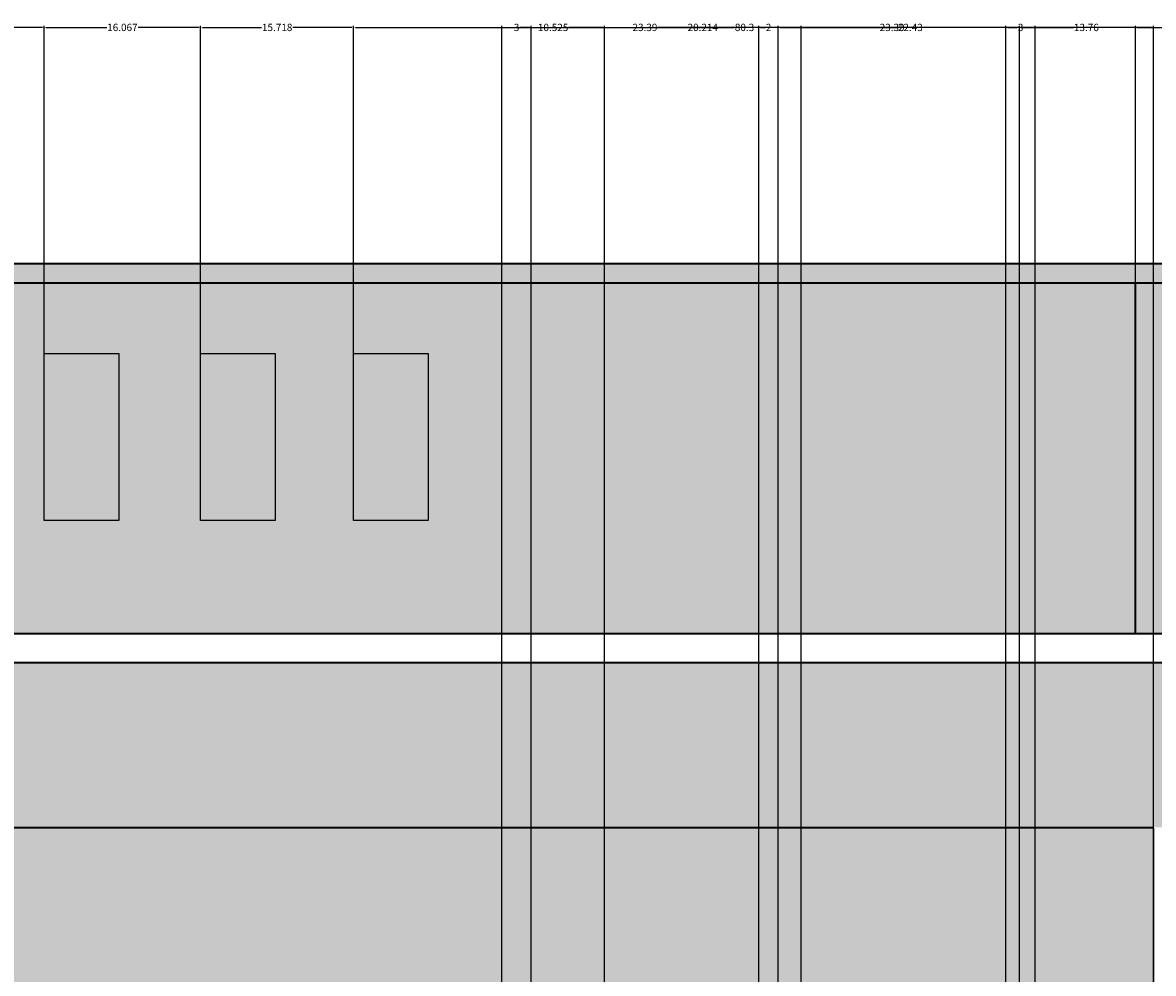
# Model space of a CAD drawing. Units: inches. Extents: x 62 to 566, y 66 to 528.
# Tile 10 of 20: x 168 to 284, y 430 to 528. Entities that reach past the tile are written whole.
import ezdxf

# ---------------------------------------------------------------- set-up
doc = ezdxf.new("R2010")
doc.units = ezdxf.units.IN
doc.header["$MEASUREMENT"] = 0
for name, color, linetype, lineweight in [('A-ANNO-DIMS', 2, 'Continuous', 18), ('A-ELEV', 7, 'Continuous', 35), ('A-GLAZ', 3, 'Continuous', 25), ('A-WALL-PATT', 8, 'Continuous', 13)]:
    doc.layers.add(name, color=color, linetype=linetype, lineweight=lineweight)
doc.styles.get("Standard").update_dxf_attribs({"font": 'arial.ttf'})
doc.dimstyles.get("Standard").update_dxf_attribs({"dimtxt": 0.75, "dimasz": 0.18, "dimexe": 0.18, "dimexo": 0.0625, "dimgap": 0.09, "dimtad": 0, "dimtih": 1, "dimtoh": 1, "dimdec": 4, "dimzin": 0, "dimdsep": 46, "dimlunit": 4, "dimtxsty": 'Standard', "dimcen": 0.09, "dimadec": 0, "dimazin": 0, "dimtfac": 1, "dimtdec": 4, "dimtofl": 0, "dimtmove": 0, "dimatfit": 3, "dimfxl": 1, "dimtolj": 1, "dimtzin": 0, "dimarcsym": 0})

# ---------------------------------------------------------------- blocks, each defined once
blk = doc.blocks.new('VENT-OPENING')
blk.add_lwpolyline([(0, 17.13), (7.66, 17.13), (7.66, 0), (0, 0)], close=True)
blk = doc.blocks.new('*D28')
at = {"layer": 'A-ANNO-DIMS', "color": 0, "lineweight": -2, "transparency": 16777216}
for p, q in [((155.59, 493.49), (155.59, 527.47)), ((170.26, 493.84), (170.26, 527.47)), ((155.77, 527.29), (161.61, 527.29)), ((170.08, 527.29), (164.25, 527.29))]:
    blk.add_line(p, q, dxfattribs=at)
at = {"layer": 'A-ANNO-DIMS', "color": 0, "transparency": 16777216}
for points in [[(155.77, 527.32), (155.77, 527.26), (155.59, 527.29)], [(170.08, 527.32), (170.08, 527.26), (170.26, 527.29)]]:
    blk.add_solid(points, dxfattribs=at)
at = {"layer": 'Defpoints', "color": 0, "transparency": 16777216}
for p in [(170.26, 527.29), (170.26, 493.78), (155.59, 493.43)]:
    blk.add_point(p, dxfattribs=at)
at = {"layer": 'A-ANNO-DIMS', "color": 0, "transparency": 16777216, "insert": (162.93, 527.29), "char_height": 0.75, "attachment_point": 5}
blk.add_mtext('\\A1;14.67', dxfattribs=at)
blk = doc.blocks.new('*D29')
at = {"layer": 'A-ANNO-DIMS', "color": 0, "lineweight": -2, "transparency": 16777216}
for p, q in [((170.26, 493.84), (170.26, 527.47)), ((186.33, 493.84), (186.33, 527.47)), ((170.44, 527.29), (176.68, 527.29)), ((186.15, 527.29), (179.91, 527.29))]:
    blk.add_line(p, q, dxfattribs=at)
at = {"layer": 'A-ANNO-DIMS', "color": 0, "transparency": 16777216}
for points in [[(170.44, 527.32), (170.44, 527.26), (170.26, 527.29)], [(186.15, 527.32), (186.15, 527.26), (186.33, 527.29)]]:
    blk.add_solid(points, dxfattribs=at)
at = {"layer": 'Defpoints', "color": 0, "transparency": 16777216}
for p in [(186.33, 527.29), (170.26, 493.78), (186.33, 493.78)]:
    blk.add_point(p, dxfattribs=at)
at = {"layer": 'A-ANNO-DIMS', "color": 0, "transparency": 16777216, "insert": (178.29, 527.29), "char_height": 0.75, "attachment_point": 5}
blk.add_mtext('\\A1;16.067', dxfattribs=at)
blk = doc.blocks.new('*D30')
at = {"layer": 'A-ANNO-DIMS', "color": 0, "lineweight": -2, "transparency": 16777216}
for p, q in [((186.33, 493.84), (186.33, 527.47)), ((202.04, 493.84), (202.04, 527.47)), ((186.51, 527.29), (192.57, 527.29)), ((201.86, 527.29), (195.8, 527.29))]:
    blk.add_line(p, q, dxfattribs=at)
at = {"layer": 'A-ANNO-DIMS', "color": 0, "transparency": 16777216}
for points in [[(186.51, 527.32), (186.51, 527.26), (186.33, 527.29)], [(201.86, 527.32), (201.86, 527.26), (202.04, 527.29)]]:
    blk.add_solid(points, dxfattribs=at)
at = {"layer": 'Defpoints', "color": 0, "transparency": 16777216}
for p in [(202.04, 527.29), (186.33, 493.78), (202.04, 493.78)]:
    blk.add_point(p, dxfattribs=at)
at = {"layer": 'A-ANNO-DIMS', "color": 0, "transparency": 16777216, "insert": (194.19, 527.29), "char_height": 0.75, "attachment_point": 5}
blk.add_mtext('\\A1;15.718', dxfattribs=at)
blk = doc.blocks.new('*D31')
at = {"layer": 'A-ANNO-DIMS', "color": 0, "lineweight": -2, "transparency": 16777216}
for p, q in [((202.04, 493.84), (202.04, 527.47)), ((282.35, 501.1), (282.35, 527.47)), ((202.22, 527.29), (241.13, 527.29)), ((282.17, 527.29), (243.26, 527.29))]:
    blk.add_line(p, q, dxfattribs=at)
at = {"layer": 'A-ANNO-DIMS', "color": 0, "transparency": 16777216}
for points in [[(202.22, 527.32), (202.22, 527.26), (202.04, 527.29)], [(282.17, 527.32), (282.17, 527.26), (282.35, 527.29)]]:
    blk.add_solid(points, dxfattribs=at)
at = {"layer": 'Defpoints', "color": 0, "transparency": 16777216}
for p in [(282.35, 527.29), (282.35, 501.04), (202.04, 493.78)]:
    blk.add_point(p, dxfattribs=at)
at = {"layer": 'A-ANNO-DIMS', "color": 0, "transparency": 16777216, "insert": (242.2, 527.29), "char_height": 0.75, "attachment_point": 5}
blk.add_mtext('\\A1;80.3', dxfattribs=at)
blk = doc.blocks.new('*D32')
at = {"layer": 'A-ANNO-DIMS', "color": 0, "lineweight": -2, "transparency": 16777216}
for p, q in [((282.35, 501.1), (282.35, 527.47)), ((416.08, 501.1), (416.08, 527.47)), ((282.53, 527.29), (347.61, 527.29)), ((415.9, 527.29), (350.83, 527.29))]:
    blk.add_line(p, q, dxfattribs=at)
at = {"layer": 'A-ANNO-DIMS', "color": 0, "transparency": 16777216}
for points in [[(282.53, 527.32), (282.53, 527.26), (282.35, 527.29)], [(415.9, 527.32), (415.9, 527.26), (416.08, 527.29)]]:
    blk.add_solid(points, dxfattribs=at)
at = {"layer": 'Defpoints', "color": 0, "transparency": 16777216}
for p in [(416.08, 527.29), (282.35, 501.04), (416.08, 501.04)]:
    blk.add_point(p, dxfattribs=at)
at = {"layer": 'A-ANNO-DIMS', "color": 0, "transparency": 16777216, "insert": (349.22, 527.29), "char_height": 0.75, "attachment_point": 5}
blk.add_mtext('\\A1;133.73', dxfattribs=at)
blk = doc.blocks.new('*D39')
at = {"layer": 'A-ANNO-DIMS', "color": 0, "lineweight": -2, "transparency": 16777216}
for p, q in [((284.2, 445.04), (284.2, 65.94)), ((217.28, 420.53), (217.28, 65.94)), ((217.46, 66.12), (249.38, 66.12)), ((284.02, 66.12), (252.1, 66.12))]:
    blk.add_line(p, q, dxfattribs=at)
at = {"layer": 'A-ANNO-DIMS', "color": 0, "transparency": 16777216}
for points in [[(217.46, 66.15), (217.46, 66.09), (217.28, 66.12)], [(284.02, 66.15), (284.02, 66.09), (284.2, 66.12)]]:
    blk.add_solid(points, dxfattribs=at)
at = {"layer": 'Defpoints', "color": 0, "transparency": 16777216}
for p in [(284.2, 445.11), (217.28, 420.6), (284.2, 66.12)]:
    blk.add_point(p, dxfattribs=at)
at = {"layer": 'A-ANNO-DIMS', "color": 0, "transparency": 16777216, "insert": (250.74, 66.12), "char_height": 0.75, "attachment_point": 5}
blk.add_mtext('\\A1;66.93', dxfattribs=at)
blk = doc.blocks.new('*D40')
at = {"layer": 'A-ANNO-DIMS', "color": 0, "lineweight": -2, "transparency": 16777216}
for p, q in [((284.2, 445.04), (284.2, 65.94)), ((316.21, 417.64), (316.21, 65.94)), ((284.38, 66.12), (298.92, 66.12)), ((316.03, 66.12), (301.49, 66.12))]:
    blk.add_line(p, q, dxfattribs=at)
at = {"layer": 'A-ANNO-DIMS', "color": 0, "transparency": 16777216}
for points in [[(284.38, 66.15), (284.38, 66.09), (284.2, 66.12)], [(316.03, 66.15), (316.03, 66.09), (316.21, 66.12)]]:
    blk.add_solid(points, dxfattribs=at)
at = {"layer": 'Defpoints', "color": 0, "transparency": 16777216}
for p in [(284.2, 445.11), (316.21, 417.71), (316.21, 66.12)]:
    blk.add_point(p, dxfattribs=at)
at = {"layer": 'A-ANNO-DIMS', "color": 0, "transparency": 16777216, "insert": (300.21, 66.12), "char_height": 0.75, "attachment_point": 5}
blk.add_mtext('\\A1;32.01', dxfattribs=at)
blk = doc.blocks.new('*D74')
at = {"layer": 'A-ANNO-DIMS', "color": 0, "lineweight": -2, "transparency": 16777216}
for p, q in [((284.2, 342.84), (284.2, 527.47)), ((304.82, 342.84), (304.82, 527.47)), ((284.38, 527.29), (292.86, 527.29)), ((304.64, 527.29), (296.16, 527.29))]:
    blk.add_line(p, q, dxfattribs=at)
at = {"layer": 'A-ANNO-DIMS', "color": 0, "transparency": 16777216}
for points in [[(284.38, 527.32), (284.38, 527.26), (284.2, 527.29)], [(304.64, 527.32), (304.64, 527.26), (304.82, 527.29)]]:
    blk.add_solid(points, dxfattribs=at)
at = {"layer": 'Defpoints', "color": 0, "transparency": 16777216}
for p in [(304.82, 527.29), (284.2, 342.78), (304.82, 342.78)]:
    blk.add_point(p, dxfattribs=at)
at = {"layer": 'A-ANNO-DIMS', "color": 0, "transparency": 16777216, "insert": (294.51, 527.29), "char_height": 0.75, "attachment_point": 5}
blk.add_mtext('\\A1;20.614', dxfattribs=at)
blk = doc.blocks.new('*D104')
at = {"layer": 'A-ANNO-DIMS', "color": 0, "lineweight": -2, "transparency": 16777216}
for p, q in [((217.28, 271.48), (217.28, 527.47)), ((220.28, 268.48), (220.28, 527.47)), ((217.46, 527.29), (218.44, 527.29)), ((220.1, 527.29), (219.11, 527.29))]:
    blk.add_line(p, q, dxfattribs=at)
at = {"layer": 'A-ANNO-DIMS', "color": 0, "transparency": 16777216}
for points in [[(217.46, 527.32), (217.46, 527.26), (217.28, 527.29)], [(220.1, 527.32), (220.1, 527.26), (220.28, 527.29)]]:
    blk.add_solid(points, dxfattribs=at)
at = {"layer": 'Defpoints', "color": 0, "transparency": 16777216}
for p in [(220.28, 527.29), (217.28, 271.41), (220.28, 268.41)]:
    blk.add_point(p, dxfattribs=at)
at = {"layer": 'A-ANNO-DIMS', "color": 0, "transparency": 16777216, "insert": (218.78, 527.29), "char_height": 0.75, "attachment_point": 5}
blk.add_mtext('\\A1;3', dxfattribs=at)
blk = doc.blocks.new('*D105')
at = {"layer": 'A-ANNO-DIMS', "color": 0, "lineweight": -2, "transparency": 16777216}
for p, q in [((220.28, 268.48), (220.28, 527.47)), ((243.67, 268.48), (243.67, 527.47)), ((220.46, 527.29), (230.61, 527.29)), ((243.49, 527.29), (233.33, 527.29))]:
    blk.add_line(p, q, dxfattribs=at)
at = {"layer": 'A-ANNO-DIMS', "color": 0, "transparency": 16777216}
for points in [[(220.46, 527.32), (220.46, 527.26), (220.28, 527.29)], [(243.49, 527.32), (243.49, 527.26), (243.67, 527.29)]]:
    blk.add_solid(points, dxfattribs=at)
at = {"layer": 'Defpoints', "color": 0, "transparency": 16777216}
for p in [(243.67, 527.29), (220.28, 268.41), (243.67, 268.41)]:
    blk.add_point(p, dxfattribs=at)
at = {"layer": 'A-ANNO-DIMS', "color": 0, "transparency": 16777216, "insert": (231.97, 527.29), "char_height": 0.75, "attachment_point": 5}
blk.add_mtext('\\A1;23.39', dxfattribs=at)
blk = doc.blocks.new('*D106')
at = {"layer": 'A-ANNO-DIMS', "color": 0, "lineweight": -2, "transparency": 16777216}
for p, q in [((243.67, 268.48), (243.67, 527.47)), ((245.67, 268.48), (245.67, 527.47)), ((243.85, 527.29), (244.33, 527.29)), ((245.49, 527.29), (245.01, 527.29))]:
    blk.add_line(p, q, dxfattribs=at)
at = {"layer": 'A-ANNO-DIMS', "color": 0, "transparency": 16777216}
for points in [[(243.85, 527.32), (243.85, 527.26), (243.67, 527.29)], [(245.49, 527.32), (245.49, 527.26), (245.67, 527.29)]]:
    blk.add_solid(points, dxfattribs=at)
at = {"layer": 'Defpoints', "color": 0, "transparency": 16777216}
for p in [(245.67, 527.29), (243.67, 268.41), (245.67, 268.41)]:
    blk.add_point(p, dxfattribs=at)
at = {"layer": 'A-ANNO-DIMS', "color": 0, "transparency": 16777216, "insert": (244.67, 527.29), "char_height": 0.75, "attachment_point": 5}
blk.add_mtext('\\A1;2', dxfattribs=at)
blk = doc.blocks.new('*D107')
at = {"layer": 'A-ANNO-DIMS', "color": 0, "lineweight": -2, "transparency": 16777216}
for p, q in [((245.67, 268.48), (245.67, 527.47)), ((269.06, 268.48), (269.06, 527.47)), ((245.85, 527.29), (256, 527.29)), ((268.88, 527.29), (258.73, 527.29))]:
    blk.add_line(p, q, dxfattribs=at)
at = {"layer": 'A-ANNO-DIMS', "color": 0, "transparency": 16777216}
for points in [[(245.85, 527.32), (245.85, 527.26), (245.67, 527.29)], [(268.88, 527.32), (268.88, 527.26), (269.06, 527.29)]]:
    blk.add_solid(points, dxfattribs=at)
at = {"layer": 'Defpoints', "color": 0, "transparency": 16777216}
for p in [(269.06, 527.29), (245.67, 268.41), (269.06, 268.41)]:
    blk.add_point(p, dxfattribs=at)
at = {"layer": 'A-ANNO-DIMS', "color": 0, "transparency": 16777216, "insert": (257.36, 527.29), "char_height": 0.75, "attachment_point": 5}
blk.add_mtext('\\A1;23.39', dxfattribs=at)
blk = doc.blocks.new('*D108')
at = {"layer": 'A-ANNO-DIMS', "color": 0, "lineweight": -2, "transparency": 16777216}
for p, q in [((269.06, 268.48), (269.06, 527.47)), ((272.06, 271.48), (272.06, 527.47)), ((269.24, 527.29), (270.22, 527.29)), ((271.88, 527.29), (270.89, 527.29))]:
    blk.add_line(p, q, dxfattribs=at)
at = {"layer": 'A-ANNO-DIMS', "color": 0, "transparency": 16777216}
for points in [[(269.24, 527.32), (269.24, 527.26), (269.06, 527.29)], [(271.88, 527.32), (271.88, 527.26), (272.06, 527.29)]]:
    blk.add_solid(points, dxfattribs=at)
at = {"layer": 'Defpoints', "color": 0, "transparency": 16777216}
for p in [(272.06, 527.29), (272.06, 271.41), (269.06, 268.41)]:
    blk.add_point(p, dxfattribs=at)
at = {"layer": 'A-ANNO-DIMS', "color": 0, "transparency": 16777216, "insert": (270.56, 527.29), "char_height": 0.75, "attachment_point": 5}
blk.add_mtext('\\A1;3', dxfattribs=at)
blk = doc.blocks.new('*D109')
at = {"layer": 'A-ANNO-DIMS', "color": 0, "lineweight": -2, "transparency": 16777216}
for p, q in [((217.28, 307.48), (217.28, 527.47)), ((227.8, 297.23), (227.8, 527.47)), ((217.46, 527.29), (220.92, 527.29)), ((227.62, 527.29), (224.15, 527.29))]:
    blk.add_line(p, q, dxfattribs=at)
at = {"layer": 'A-ANNO-DIMS', "color": 0, "transparency": 16777216}
for points in [[(217.46, 527.32), (217.46, 527.26), (217.28, 527.29)], [(227.62, 527.32), (227.62, 527.26), (227.8, 527.29)]]:
    blk.add_solid(points, dxfattribs=at)
at = {"layer": 'Defpoints', "color": 0, "transparency": 16777216}
for p in [(227.8, 527.29), (217.28, 307.41), (227.8, 297.17)]:
    blk.add_point(p, dxfattribs=at)
at = {"layer": 'A-ANNO-DIMS', "color": 0, "transparency": 16777216, "insert": (222.54, 527.29), "char_height": 0.75, "attachment_point": 5}
blk.add_mtext('\\A1;10.525', dxfattribs=at)
blk = doc.blocks.new('*D110')
at = {"layer": 'A-ANNO-DIMS', "color": 0, "lineweight": -2, "transparency": 16777216}
for p, q in [((227.8, 297.23), (227.8, 527.47)), ((248.01, 297.23), (248.01, 527.47)), ((227.98, 527.29), (236.26, 527.29)), ((247.83, 527.29), (239.56, 527.29))]:
    blk.add_line(p, q, dxfattribs=at)
at = {"layer": 'A-ANNO-DIMS', "color": 0, "transparency": 16777216}
for points in [[(227.98, 527.32), (227.98, 527.26), (227.8, 527.29)], [(247.83, 527.32), (247.83, 527.26), (248.01, 527.29)]]:
    blk.add_solid(points, dxfattribs=at)
at = {"layer": 'Defpoints', "color": 0, "transparency": 16777216}
for p in [(248.01, 527.29), (227.8, 297.17), (248.01, 297.17)]:
    blk.add_point(p, dxfattribs=at)
at = {"layer": 'A-ANNO-DIMS', "color": 0, "transparency": 16777216, "insert": (237.91, 527.29), "char_height": 0.75, "attachment_point": 5}
blk.add_mtext('\\A1;20.214', dxfattribs=at)
blk = doc.blocks.new('*D111')
at = {"layer": 'A-ANNO-DIMS', "color": 0, "lineweight": -2, "transparency": 16777216}
for p, q in [((248.01, 297.23), (248.01, 527.47)), ((270.44, 297.23), (270.44, 527.47)), ((248.19, 527.29), (257.87, 527.29)), ((270.26, 527.29), (260.59, 527.29))]:
    blk.add_line(p, q, dxfattribs=at)
at = {"layer": 'A-ANNO-DIMS', "color": 0, "transparency": 16777216}
for points in [[(248.19, 527.32), (248.19, 527.26), (248.01, 527.29)], [(270.26, 527.32), (270.26, 527.26), (270.44, 527.29)]]:
    blk.add_solid(points, dxfattribs=at)
at = {"layer": 'Defpoints', "color": 0, "transparency": 16777216}
for p in [(270.44, 527.29), (248.01, 297.17), (270.44, 297.17)]:
    blk.add_point(p, dxfattribs=at)
at = {"layer": 'A-ANNO-DIMS', "color": 0, "transparency": 16777216, "insert": (259.23, 527.29), "char_height": 0.75, "attachment_point": 5}
blk.add_mtext('\\A1;22.43', dxfattribs=at)
blk = doc.blocks.new('*D112')
at = {"layer": 'A-ANNO-DIMS', "color": 0, "lineweight": -2, "transparency": 16777216}
for p, q in [((270.44, 297.23), (270.44, 527.47)), ((284.2, 307.48), (284.2, 527.47)), ((270.62, 527.29), (276, 527.29)), ((284.02, 527.29), (278.64, 527.29))]:
    blk.add_line(p, q, dxfattribs=at)
at = {"layer": 'A-ANNO-DIMS', "color": 0, "transparency": 16777216}
for points in [[(270.62, 527.32), (270.62, 527.26), (270.44, 527.29)], [(284.02, 527.32), (284.02, 527.26), (284.2, 527.29)]]:
    blk.add_solid(points, dxfattribs=at)
at = {"layer": 'Defpoints', "color": 0, "transparency": 16777216}
for p in [(284.2, 527.29), (284.2, 307.41), (270.44, 297.17)]:
    blk.add_point(p, dxfattribs=at)
at = {"layer": 'A-ANNO-DIMS', "color": 0, "transparency": 16777216, "insert": (277.32, 527.29), "char_height": 0.75, "attachment_point": 5}
blk.add_mtext('\\A1;13.76', dxfattribs=at)

msp = doc.modelspace()

# ---------------------------------------------------------------- hatches: boundary and pattern name
at = {"layer": 'A-WALL-PATT'}
h = msp.add_hatch(color=256, dxfattribs=at)
h.dxf.hatch_style = 1
h.paths.add_polyline_path([(416.0836, 462.0423), (125.9418, 462.0423), (125.9418, 414.3686), (125.9418, 270.3686), (125.9418, 126.3686), (142.3851, 126.3686), (142.3851, 270.3686), (142.3851, 414.3686), (142.3851, 445.1064), (284.2021, 445.1064), (416.0836, 445.1064)])
h.paths.add_polyline_path([(435.3945, 503.0423), (426.3652, 503.0423), (120.4058, 503.0423), (120.4058, 501.0423), (125.9418, 501.0423), (416.0836, 501.0423), (426.3652, 501.0423), (430.6938, 501.0423), (435.3945, 501.0423)])
h.paths.add_polyline_path([(439.6878, 352.4848), (392.4793, 352.4848), (392.4793, 307.4128), (217.2752, 307.4128), (217.2752, 295.4098), (217.2752, 271.4128), (272.0586, 271.4128), (439.6878, 271.4128)])
h.paths.add_polyline_path([(248.0143, 297.1682), (255.6783, 297.1682), (255.6783, 280.0423), (248.0143, 280.0423)], flags=16)
h.paths.add_polyline_path([(235.4641, 280.0423), (227.8001, 280.0423), (227.8001, 297.1682), (235.4641, 297.1682)], flags=16)
h.paths.add_polyline_path([(270.4427, 297.1682), (278.1067, 297.1682), (278.1067, 280.0423), (270.4427, 280.0423)], flags=16)
h.paths.add_polyline_path([(296.3755, 297.1682), (304.0395, 297.1682), (304.0395, 280.0423), (296.3755, 280.0423)], flags=16)
h.paths.add_polyline_path([(319.2543, 297.1682), (326.9183, 297.1682), (326.9183, 280.0423), (319.2543, 280.0423)], flags=16)
h.paths.add_polyline_path([(341.2622, 297.1682), (348.9262, 297.1682), (348.9262, 280.0423), (341.2622, 280.0423)], flags=16)
h.paths.add_polyline_path([(389.2857, 298.3985), (433.8102, 298.3985), (433.8102, 294.9497), (389.2857, 294.9497)], flags=16)
h.paths.add_polyline_path([(389.2857, 291.6038), (433.8102, 291.6038), (433.8102, 288.155), (389.2857, 288.155)], flags=16)
h.paths.add_polyline_path([(389.2857, 284.9607), (433.8102, 284.9607), (433.8102, 281.5119), (389.2857, 281.5119)], flags=16)
h.paths.add_polyline_path([(403.5849, 311.4736), (403.5849, 317.4388), (433.1636, 317.4388), (433.1636, 311.4736)], flags=16)
h.paths.add_polyline_path([(403.5849, 323.1329), (403.5849, 329.0982), (433.1636, 329.0982), (433.1636, 323.1329)], flags=16)
h.paths.add_polyline_path([(403.5849, 334.5211), (403.5849, 340.4863), (433.1636, 340.4863), (433.1636, 334.5211)], flags=16)
h.paths.add_polyline_path([(272.0586, 160.3545), (217.2752, 160.3545), (217.2752, 129.0504), (217.2752, 126.3686), (272.0586, 126.3686)], flags=17)
h.paths.add_polyline_path([(220.5897, 149.5749), (220.5897, 152.296), (267.7931, 152.296), (267.7931, 149.5749)], flags=16)
h.paths.add_polyline_path([(267.7931, 146.6724), (267.7931, 143.9513), (220.5897, 143.9513), (220.5897, 146.6724)], flags=16)
h.paths.add_polyline_path([(220.5897, 155.3799), (220.5897, 158.101), (267.7931, 158.101), (267.7931, 155.3799)], flags=16)
h.paths.add_polyline_path([(267.7931, 140.686), (267.7931, 137.9649), (220.5897, 137.9649), (220.5897, 140.686)], flags=16)
h.paths.add_polyline_path([(267.7931, 135.516), (267.7931, 132.7949), (220.5897, 132.7949), (220.5897, 135.516)], flags=16)
h = msp.add_hatch(dxfattribs=at)
h.set_pattern_fill('ANSI36', color=256, scale=8.8)
h.paths.add_polyline_path([(217.2752, 420.597), (169.0431, 420.597), (169.0431, 126.3686), (217.2752, 126.3686), (217.2752, 129.0504), (217.2752, 271.4128), (217.2752, 295.4128), (217.2752, 307.4128)])
h.paths.add_polyline_path([(282.3509, 501.0423), (125.9418, 501.0423), (125.9418, 465.0423), (282.3509, 465.0423)])
h.paths.add_polyline_path([(209.709, 476.6506), (202.045, 476.6506), (202.045, 493.7764), (209.709, 493.7764)], flags=16)
h.paths.add_polyline_path([(193.9913, 476.6506), (186.3273, 476.6506), (186.3273, 493.7764), (193.9913, 493.7764)], flags=16)
h.paths.add_polyline_path([(177.9243, 476.6506), (170.2603, 476.6506), (170.2603, 493.7764), (177.9243, 493.7764)], flags=16)
h.paths.add_polyline_path([(163.2545, 476.3015), (155.5905, 476.3015), (155.5905, 493.4274), (163.2545, 493.4274)], flags=16)
h.paths.add_polyline_path([(148.2354, 476.3015), (140.5713, 476.3015), (140.5713, 493.4274), (148.2354, 493.4274)], flags=16)
h.paths.add_polyline_path([(284.2021, 126.3686), (87.8962, 126.3686), (87.8962, 114.3686), (87.8962, 90.3686), (284.2021, 90.3686)])
h.paths.add_polyline_path([(474.1214, 126.3686), (396.433, 126.3686), (396.433, 90.3686), (474.1214, 90.3686)])
h = msp.add_hatch(color=256, dxfattribs=at)
h.dxf.hatch_style = 1
h.paths.add_polyline_path([(416.0836, 501.0423), (282.3509, 501.0423), (282.3509, 465.0423), (416.0836, 465.0423)])
h.paths.add_polyline_path([(284.2021, 420.597), (272.0586, 420.597), (272.0586, 309.5388), (272.0586, 307.4128), (284.2021, 307.4128)], flags=17)
h.paths.add_polyline_path([(284.2021, 445.1064), (142.3851, 445.1064), (142.3851, 414.3686), (142.3851, 270.3686), (142.3851, 126.3686), (163.6548, 126.3686), (163.6548, 270.5016), (163.6548, 414.5016), (163.6548, 427.4752), (284.2021, 427.4752)])
h.paths.add_polyline_path([(235.4641, 297.1682), (227.8001, 297.1682), (227.8001, 280.0423), (235.4641, 280.0423)], flags=17)
h.paths.add_polyline_path([(255.6783, 297.1682), (248.0143, 297.1682), (248.0143, 280.0423), (255.6783, 280.0423)], flags=17)
h.paths.add_polyline_path([(278.1067, 297.1682), (270.4427, 297.1682), (270.4427, 280.0423), (278.1067, 280.0423)], flags=17)
h.paths.add_polyline_path([(304.0395, 297.1682), (296.3755, 297.1682), (296.3755, 280.0423), (304.0395, 280.0423)])
h.paths.add_polyline_path([(326.9183, 297.1682), (319.2543, 297.1682), (319.2543, 280.0423), (326.9183, 280.0423)])
h.paths.add_polyline_path([(348.9262, 297.1682), (341.2622, 297.1682), (341.2622, 280.0423), (348.9262, 280.0423)])
h.paths.add_polyline_path([(433.8102, 284.9607), (389.2857, 284.9607), (389.2857, 281.5119), (433.8102, 281.5119)])
h.paths.add_polyline_path([(433.8102, 291.6038), (389.2857, 291.6038), (389.2857, 288.155), (433.8102, 288.155)])
h.paths.add_polyline_path([(433.8102, 298.3985), (389.2857, 298.3985), (389.2857, 294.9497), (433.8102, 294.9497)])
h.paths.add_polyline_path([(433.1636, 317.4388), (403.5849, 317.4388), (403.5849, 311.4736), (433.1636, 311.4736)])
h.paths.add_polyline_path([(433.1636, 329.0982), (403.5849, 329.0982), (403.5849, 323.1329), (433.1636, 323.1329)])
h.paths.add_polyline_path([(433.1636, 340.4863), (403.5849, 340.4863), (403.5849, 334.5211), (433.1636, 334.5211)])
h.paths.add_polyline_path([(284.2021, 271.4128), (272.0586, 271.4128), (272.0586, 160.3545), (272.0586, 126.3686), (284.2021, 126.3686)])
h.paths.add_polyline_path([(267.7931, 158.101), (220.5897, 158.101), (220.5897, 155.3799), (267.7931, 155.3799)], flags=17)
h.paths.add_polyline_path([(267.7931, 152.296), (220.5897, 152.296), (220.5897, 149.5749), (267.7931, 149.5749)], flags=17)
h.paths.add_polyline_path([(267.7931, 146.6724), (220.5897, 146.6724), (220.5897, 143.9513), (267.7931, 143.9513)], flags=17)
h.paths.add_polyline_path([(267.7931, 140.686), (220.5897, 140.686), (220.5897, 137.9649), (267.7931, 137.9649)], flags=17)
h.paths.add_polyline_path([(267.7931, 135.516), (220.5897, 135.516), (220.5897, 132.7949), (267.7931, 132.7949)], flags=17)
h.paths.add_polyline_path([(148.2354, 493.4274), (140.5713, 493.4274), (140.5713, 476.3015), (148.2354, 476.3015)])
h.paths.add_polyline_path([(163.2545, 493.4274), (155.5905, 493.4274), (155.5905, 476.3015), (163.2545, 476.3015)])
h.paths.add_polyline_path([(177.9243, 493.7764), (170.2603, 493.7764), (170.2603, 476.6506), (177.9243, 476.6506)])
h.paths.add_polyline_path([(193.9913, 493.7764), (186.3273, 493.7764), (186.3273, 476.6506), (193.9913, 476.6506)])
h.paths.add_polyline_path([(209.709, 493.7764), (202.045, 493.7764), (202.045, 476.6506), (209.709, 476.6506)])

# ---------------------------------------------------------------- linework, layer by layer
at = {"layer": 'A-ELEV'}
for p, q in [((120.4058, 503.0423), (426.3652, 503.0423)), ((125.9418, 501.0423), (416.0836, 501.0423)), ((282.3509, 465.0423), (282.3509, 501.0423)), ((125.9418, 465.0423), (416.0836, 465.0423)), ((125.9418, 462.0423), (416.0836, 462.0423)), ((142.3851, 445.1064), (284.2021, 445.1064))]:
    msp.add_line(p, q, dxfattribs=at)

# ---------------------------------------------------------------- block references
at = {"layer": 'A-GLAZ'}
for p in [(170.2603, 476.6506), (186.3273, 476.6506), (202.045, 476.6506)]:
    msp.add_blockref('VENT-OPENING', p, dxfattribs=at)

# ---------------------------------------------------------------- dimensions: what is measured, and where the dimension line sits
at = {"layer": 'A-ANNO-DIMS'}
for base, p1, p2, override, picture, middle in [((170.2603, 527.2923), (155.5905, 493.4274), (170.2603, 493.7764), {"dimdec": 2, "dimlfac": 1, "dimrnd": 0, "dimzin": 0, "dimdsep": 46, "dimlunit": 2}, '*D28', (162.9254, 527.2923)), ((186.3273, 527.2923), (170.2603, 493.7764), (186.3273, 493.7764), {"dimdec": 3, "dimlfac": 1, "dimrnd": 0, "dimzin": 0, "dimdsep": 46, "dimlunit": 2}, '*D29', (178.2938, 527.2923)), ((202.045, 527.2923), (186.3273, 493.7764), (202.045, 493.7764), {"dimdec": 3, "dimlfac": 1, "dimrnd": 0, "dimzin": 0, "dimdsep": 46, "dimlunit": 2}, '*D30', (194.1861, 527.2923)), ((282.3509, 527.2923), (202.045, 493.7764), (282.3509, 501.0423), {"dimdec": 1, "dimlfac": 1, "dimrnd": 0, "dimzin": 0, "dimdsep": 46, "dimlunit": 2}, '*D31', (242.1979, 527.2923)), ((220.2752, 527.2923), (217.2752, 271.4128), (220.2752, 268.4128), {"dimdec": 0, "dimlfac": 1, "dimrnd": 0, "dimzin": 0, "dimdsep": 46, "dimlunit": 2}, '*D104', (218.7752, 527.2923)), ((227.8001, 527.2923), (217.2752, 307.4128), (227.8001, 297.1682), {"dimdec": 3, "dimlfac": 1, "dimrnd": 0, "dimzin": 0, "dimdsep": 46, "dimlunit": 2}, '*D109', (222.5377, 527.2923)), ((243.6669, 527.2923), (220.2752, 268.4128), (243.6669, 268.4128), {"dimdec": 2, "dimlfac": 1, "dimrnd": 0, "dimzin": 0, "dimdsep": 46, "dimlunit": 2}, '*D105', (231.971, 527.2923)), ((248.0143, 527.2923), (227.8001, 297.1682), (248.0143, 297.1682), {"dimdec": 3, "dimlfac": 1, "dimrnd": 0, "dimzin": 0, "dimdsep": 46, "dimlunit": 2}, '*D110', (237.9072, 527.2923)), ((245.6669, 527.2923), (243.6669, 268.4128), (245.6669, 268.4128), {"dimdec": 0, "dimlfac": 1, "dimrnd": 0, "dimzin": 0, "dimdsep": 46, "dimlunit": 2}, '*D106', (244.6669, 527.2923)), ((269.0586, 527.2923), (245.6669, 268.4128), (269.0586, 268.4128), {"dimdec": 2, "dimlfac": 1, "dimrnd": 0, "dimzin": 0, "dimdsep": 46, "dimlunit": 2}, '*D107', (257.3627, 527.2923)), ((270.4427, 527.2923), (248.0143, 297.1682), (270.4427, 297.1682), {"dimdec": 2, "dimlfac": 1, "dimrnd": 0, "dimzin": 0, "dimdsep": 46, "dimlunit": 2}, '*D111', (259.2285, 527.2923)), ((272.0586, 527.2923), (269.0586, 268.4128), (272.0586, 271.4128), {"dimdec": 0, "dimlfac": 1, "dimrnd": 0, "dimzin": 0, "dimdsep": 46, "dimlunit": 2}, '*D108', (270.5586, 527.2923)), ((284.2021, 527.2923), (270.4427, 297.1682), (284.2021, 307.4128), {"dimdec": 2, "dimlfac": 1, "dimrnd": 0, "dimzin": 0, "dimdsep": 46, "dimlunit": 2}, '*D112', (277.3224, 527.2923)), ((416.0836, 527.2923), (282.3509, 501.0423), (416.0836, 501.0423), {"dimdec": 2, "dimlfac": 1, "dimrnd": 0, "dimzin": 0, "dimdsep": 46, "dimlunit": 2}, '*D32', (349.2172, 527.2923)), ((304.8163, 527.2923), (284.2021, 342.7821), (304.8163, 342.7821), {"dimdec": 3, "dimlfac": 1, "dimrnd": 0, "dimzin": 0, "dimdsep": 46, "dimlunit": 2}, '*D74', (294.5092, 527.2923)), ((284.2021, 66.1186), (217.2752, 420.597), (284.2021, 445.1064), {"dimdec": 2, "dimlfac": 1, "dimrnd": 0, "dimzin": 0, "dimdsep": 46, "dimlunit": 2}, '*D39', (250.7386, 66.1186)), ((316.2101, 66.1186), (284.2021, 445.1064), (316.2101, 417.7059), {"dimdec": 2, "dimlfac": 1, "dimrnd": 0, "dimzin": 0, "dimdsep": 46, "dimlunit": 2}, '*D40', (300.2061, 66.1186))]:
    dim = msp.add_linear_dim(base=base, p1=p1, p2=p2, dimstyle='Standard', override=override, dxfattribs=at)
    dim.commit()
    dim.dimension.update_dxf_attribs({"geometry": picture, "text_midpoint": middle})

doc.saveas('drawing.dxf')
